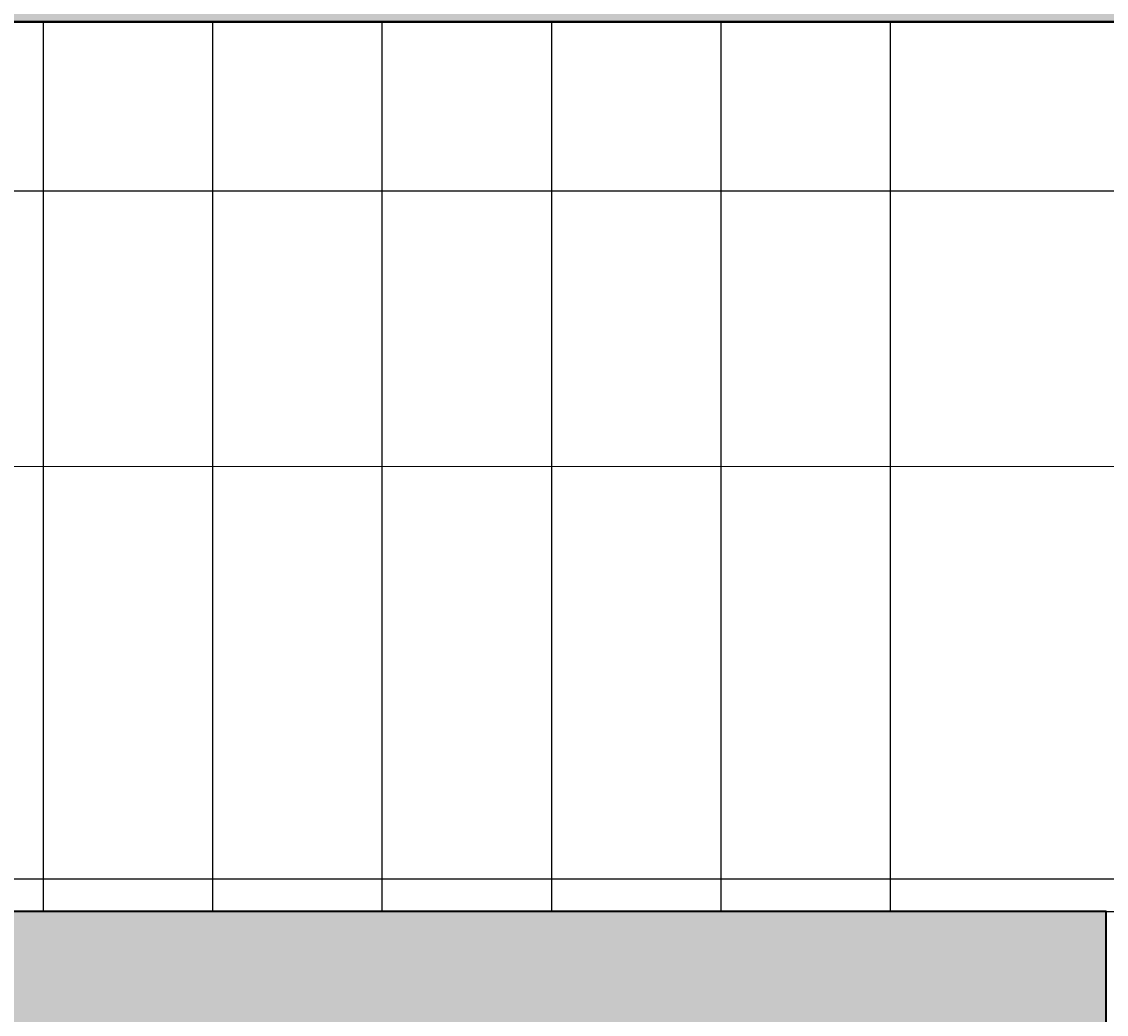
# Model space of a CAD drawing. Units: inches. Extents: x 1998 to 2588, y 1139 to 1977.
# Tile 108 of 134: x 2447 to 2498, y 1590 to 1637. Entities that reach past the tile are written whole.
import ezdxf

# ---------------------------------------------------------------- set-up
doc = ezdxf.new("R2010")
doc.units = ezdxf.units.IN
for name, color, linetype, lineweight in [('A-ANNO-DIMS', 2, 'Continuous', 18), ('A-ANNO-SYMB', 7, 'Continuous', 18), ('A-FLOR-EVTR', 7, 'Continuous', 35), ('A-FLOR-STRS', 7, 'Continuous', 25), ('A-WALL-PATT', 252, 'Continuous', 13), ('WALL', 200, 'Continuous', 35)]:
    doc.layers.add(name, color=color, linetype=linetype, lineweight=lineweight)
doc.styles.get("Standard").update_dxf_attribs({"font": 'arial.ttf'})
doc.dimstyles.get("Standard").update_dxf_attribs({"dimtxt": 0.18, "dimasz": 0.18, "dimexe": 0.18, "dimexo": 0.0625, "dimgap": 0.09, "dimtad": 0, "dimtih": 1, "dimtoh": 1, "dimdec": 4, "dimzin": 0, "dimdsep": 46, "dimtxsty": 'Standard', "dimcen": 0.09, "dimadec": 0, "dimazin": 0, "dimtfac": 1, "dimtdec": 4, "dimtofl": 0, "dimtmove": 0, "dimatfit": 3, "dimfxl": 1, "dimtolj": 1, "dimtzin": 0, "dimarcsym": 0})

# ---------------------------------------------------------------- blocks, each defined once
blk = doc.blocks.new('*D24')
at = {"layer": 'A-ANNO-DIMS', "color": 0, "lineweight": -2, "transparency": 16777216}
for p, q in [((2398.535, 1911.232), (2588.309, 1911.232)), ((2588.129, 1911.052), (2588.129, 1570.164)), ((2588.129, 1228.912), (2588.129, 1569.8)), ((2527.535, 1228.732), (2588.309, 1228.732))]:
    blk.add_line(p, q, dxfattribs=at)
at = {"layer": 'A-ANNO-DIMS', "color": 0, "transparency": 16777216}
for points in [[(2588.099, 1911.052), (2588.159, 1911.052), (2588.129, 1911.232)], [(2588.099, 1228.912), (2588.159, 1228.912), (2588.129, 1228.732)]]:
    blk.add_solid(points, dxfattribs=at)
at = {"layer": 'Defpoints', "color": 0, "transparency": 16777216}
for p in [(2398.473, 1911.232), (2588.129, 1911.232), (2527.473, 1228.732)]:
    blk.add_point(p, dxfattribs=at)
at = {"layer": 'A-ANNO-DIMS', "color": 0, "transparency": 16777216, "insert": (2588.129, 1569.982), "char_height": 0.18, "attachment_point": 5}
blk.add_mtext('\\A1;682.5', dxfattribs=at)
blk = doc.blocks.new('*D39')
at = {"layer": 'A-ANNO-DIMS', "color": 0, "lineweight": -2, "transparency": 16777216}
for p, q in [((2115.035, 1628.742), (2588.309, 1628.742)), ((2588.129, 1628.562), (2588.129, 1612.685)), ((2588.129, 1596.444), (2588.129, 1612.321)), ((2115.035, 1596.264), (2588.309, 1596.264))]:
    blk.add_line(p, q, dxfattribs=at)
at = {"layer": 'A-ANNO-DIMS', "color": 0, "transparency": 16777216}
for points in [[(2588.099, 1628.562), (2588.159, 1628.562), (2588.129, 1628.742)], [(2588.099, 1596.444), (2588.159, 1596.444), (2588.129, 1596.264)]]:
    blk.add_solid(points, dxfattribs=at)
at = {"layer": 'Defpoints', "color": 0, "transparency": 16777216}
for p in [(2114.973, 1628.742), (2588.129, 1628.742), (2114.973, 1596.264)]:
    blk.add_point(p, dxfattribs=at)
at = {"layer": 'A-ANNO-DIMS', "color": 0, "transparency": 16777216, "insert": (2588.129, 1612.503), "char_height": 0.18, "attachment_point": 5}
blk.add_mtext('\\A1;32.48', dxfattribs=at)

msp = doc.modelspace()

# ---------------------------------------------------------------- hatches: boundary and pattern name
at = {"layer": 'A-WALL-PATT'}
h = msp.add_hatch(color=256, dxfattribs=at)
h.dxf.hatch_style = 1
h.paths.add_polyline_path([(2527.4729, 1362.2324), (2510.9729, 1362.2324), (2510.9729, 1357.7324), (2518.4729, 1357.7324), (2518.4729, 1237.7324), (2503.1458, 1237.7324), (2503.1458, 1228.7324), (2527.4729, 1228.7324)])
h.paths.add_polyline_path([(2490.5682, 1362.2324), (2398.4729, 1362.2324), (2398.4729, 1357.7324), (2490.5682, 1357.7324)])
h.paths.add_polyline_path([(2224.9729, 1264.7324), (2222.9729, 1264.7324), (2222.9729, 1232.4125), (2341.4729, 1232.4125), (2341.4729, 1234.4125), (2224.9729, 1234.4125)])
h.paths.add_polyline_path([(2334.5332, 1273.7324), (2264.7638, 1273.7324), (2264.7638, 1269.5611, -0.043659), (2264.3413, 1264.7324), (2334.5332, 1264.7324)])
h.paths.add_polyline_path([(2236.9551, 1273.7324), (2234.4125, 1273.7324), (2234.4125, 1264.7324), (2236.9551, 1264.7324), (2236.9551, 1269.5611)])
h.paths.add_polyline_path([(2222.9729, 1293.2324), (2096.9729, 1293.2324), (2096.9729, 1345.0966), (2087.9729, 1345.0966), (2087.9729, 1284.2324), (2222.9729, 1284.2324), (2222.9729, 1285.137)])
h.paths.add_polyline_path([(2096.9729, 1458.7927), (2087.9729, 1458.7927), (2087.9729, 1417.7324), (2087.9729, 1413.2324), (2096.9729, 1413.2324), (2096.9729, 1417.7324)])
h.paths.add_polyline_path([(2096.9729, 1413.2324), (2087.9729, 1413.2324), (2087.9729, 1365.5012), (2096.9729, 1365.5012), (2096.9729, 1369.3358)])
h.paths.add_polyline_path([(2186.2943, 1417.7324), (2138.6074, 1417.7324), (2096.9729, 1417.7324), (2096.9729, 1413.2324), (2138.6074, 1413.2324), (2186.2943, 1413.2324)])
h.paths.add_polyline_path([(2181.4729, 1465.7324), (2176.9729, 1465.7324), (2176.9729, 1451.6434), (2181.4729, 1451.6434)])
h.paths.add_polyline_path([(2181.4729, 1422.1664), (2176.9729, 1422.1664), (2176.9729, 1417.7324), (2181.4729, 1417.7324)])
h.paths.add_polyline_path([(2063.9729, 1465.7324), (2087.9729, 1465.7324), (2087.9729, 1470.2324), (2059.4729, 1470.2324), (2059.4729, 1413.2324), (2087.9729, 1413.2324), (2087.9729, 1417.7324), (2063.9729, 1417.7324)])
h.paths.add_polyline_path([(2181.4729, 1755.2324), (2176.9729, 1755.2324), (2176.9729, 1748.6798), (2177.0513, 1748.6798), (2181.4729, 1748.6798)])
h.paths.add_polyline_path([(2227.4729, 1707.2324), (2220.4647, 1707.2324), (2220.4647, 1702.7324), (2222.9729, 1702.7324), (2222.9729, 1604.637), (2227.4729, 1604.637)])
h.paths.add_polyline_path([(2114.9729, 1702.7324), (2105.9729, 1702.7324), (2105.9729, 1628.4781, -0.0318759), (2110.1012, 1628.7416), (2114.9729, 1628.7416)])
h.paths.add_polyline_path([(2345.9729, 1739.3278), (2341.4729, 1739.3278), (2341.4729, 1647.5211), (2345.9729, 1647.5211)])
h.paths.add_polyline_path([(2350.6273, 1641.2324), (2345.9729, 1641.2324), (2345.9729, 1636.7324), (2350.6273, 1636.7324), (2350.6273, 1639.8729)])
h.paths.add_polyline_path([(2501.9729, 1641.2324), (2407.9729, 1641.2324), (2392.5005, 1641.2324), (2392.5005, 1639.8729), (2392.5005, 1636.7324), (2501.9729, 1636.7324)])
h.paths.add_polyline_path([(2510.9729, 1755.2324), (2501.9729, 1755.2324), (2501.9729, 1641.2324), (2510.9729, 1641.2324)])
h.paths.add_polyline_path([(2549.1786, 1641.2324), (2522.3775, 1641.2324), (2522.3775, 1636.7324), (2540.1786, 1636.7324), (2540.1786, 1480.7324), (2522.3775, 1480.7324), (2522.3775, 1476.2324), (2549.1786, 1476.2324)])
h.paths.add_polyline_path([(2498.1786, 1594.7324), (2407.9729, 1594.7324), (2407.9729, 1585.7324), (2416.9729, 1585.7324), (2489.1786, 1585.7324), (2489.1786, 1531.7324), (2416.9729, 1531.7324), (2407.9729, 1531.7324), (2407.9729, 1522.7324), (2498.1786, 1522.7324)])
h.paths.add_polyline_path([(2351.6437, 1480.7324), (2345.9729, 1480.7324), (2345.9729, 1476.2324), (2351.6437, 1476.2324), (2351.6437, 1477.5919)])
h.paths.add_polyline_path([(2501.9729, 1480.7324), (2498.1786, 1480.7324), (2407.9729, 1480.7324), (2393.5168, 1480.7324), (2393.5168, 1477.5919), (2393.5168, 1476.2324), (2501.9729, 1476.2324)])

# ---------------------------------------------------------------- linework, layer by layer
at = {"layer": 'A-ANNO-SYMB'}
msp.add_line((2407.9729, 1615.7324), (2505.7676, 1615.7324), dxfattribs=at)
at = {"layer": 'A-FLOR-EVTR'}
msp.add_lwpolyline([(2407.9729, 1522.7324), (2498.1786, 1522.7324), (2498.1786, 1594.7324), (2407.9729, 1594.7324)], close=True, dxfattribs=at)
at = {"layer": 'A-FLOR-STRS'}
for p, q in [((2447.9729, 1636.7324), (2447.9729, 1594.7324)), ((2455.9729, 1636.7324), (2455.9729, 1594.7324)), ((2463.9729, 1636.7324), (2463.9729, 1594.7324)), ((2471.9729, 1636.7324), (2471.9729, 1594.7324)), ((2479.9729, 1636.7324), (2479.9729, 1594.7324)), ((2487.9729, 1636.7324), (2487.9729, 1594.7324)), ((2407.9729, 1594.7324), (2540.1786, 1594.7324))]:
    msp.add_line(p, q, dxfattribs=at)
at = {"layer": 'WALL'}
for p, q in [((2501.9729, 1636.7324), (2392.5005, 1636.7324)), ((2407.9729, 1636.7324), (2501.9729, 1636.7324))]:
    msp.add_line(p, q, dxfattribs=at)

# ---------------------------------------------------------------- dimensions: what is measured, and where the dimension line sits
at = {"layer": 'A-ANNO-DIMS'}
for base, p1, p2, override, picture, middle in [((2588.1286, 1911.2324), (2527.4729, 1228.7324), (2398.4729, 1911.2324), {"dimdec": 1, "dimlfac": 1, "dimrnd": 0, "dimzin": 0, "dimdsep": 46, "dimlunit": 2}, '*D24', (2588.1286, 1569.9824)), ((2588.1286, 1628.7416), (2114.9729, 1596.2642), (2114.9729, 1628.7416), {"dimdec": 2, "dimlfac": 1, "dimrnd": 0, "dimzin": 0, "dimdsep": 46, "dimlunit": 2}, '*D39', (2588.1286, 1612.5029))]:
    dim = msp.add_linear_dim(base=base, p1=p1, p2=p2, angle=90, dimstyle='Standard', override=override, dxfattribs=at)
    dim.commit()
    dim.dimension.update_dxf_attribs({"geometry": picture, "text_midpoint": middle})

doc.saveas('drawing.dxf')
